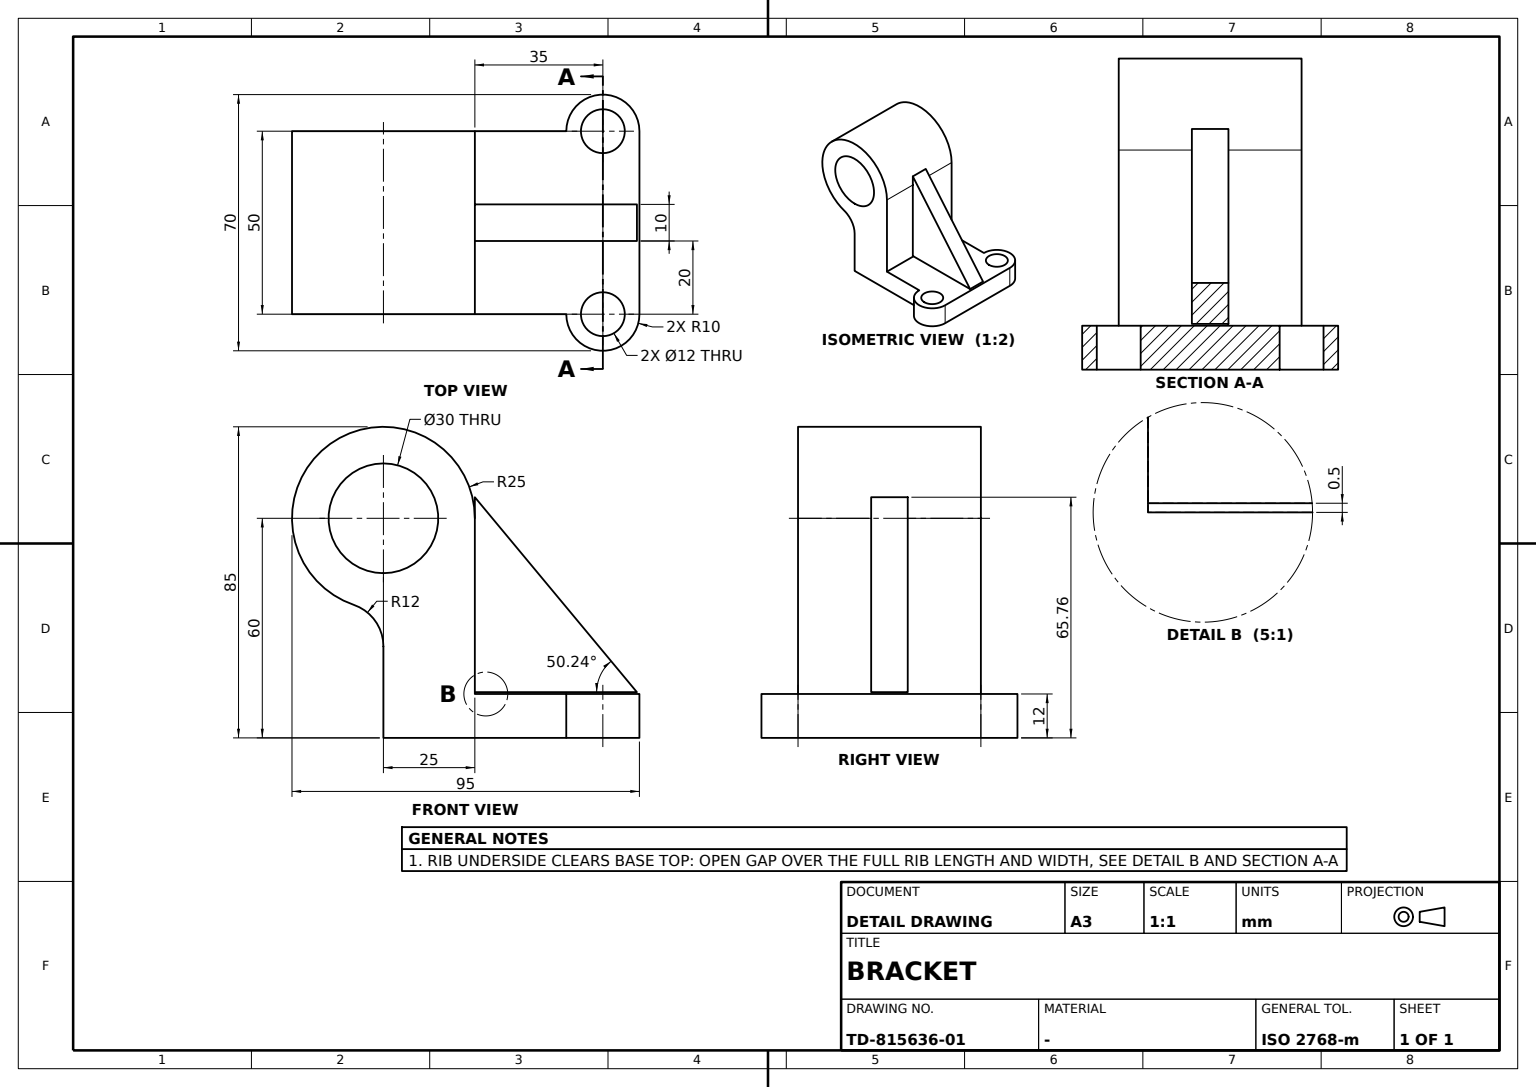
CATIA V5 part; units mm, degrees
sketch "Sketch1" plane through (0, 0, 0) normal (1, 0, 0) x (0, 1, 0)
  point P0 (0, 54)
  line L0 (0, 54) -> (0, 6)
  line L1 (0, 6) -> (45, 6)
  point P1 (45, 6)
  line L2 (45, 6) -> (45, -6)
  point P2 (45, -6)
  line L3 (45, -6) -> (-25, -6)
  line L4 (-25, -6) -> (-25, 19)
  point P3 (-25, 54)
  circle A0 centre (-25, 54) radius 15
  arc A1 (0, 54) -> (-33.1081, 30.3514) centre (-25, 54) ccw
  point P4 (0, 54)
  arc A2 (-33.1081, 30.3514) -> (-25, 19) centre (-37, 19) cw
  point P5 (0, 54)
  dimension "length L2" = 12
  dimension "distance L4 L0" = 25
  dimension "length L3" = 70
  dimension "radius A1" = 25
  dimension "radius A0" = 15
  dimension "radius A2" = 12
  dimension "distance P3 L3" = 60
  constraint vertical L0 y-axis
  constraint vertical L2 y-axis
  constraint vertical L4 y-axis
  constraint horizontal L1 x-axis
  constraint horizontal L3 x-axis
  constraint coincidence A1 P4
  constraint coincidence P4 y-axis
  constraint coincidence L4 P3
  constraint coincidence P4 P0
  constraint coincidence P0 P5
  constraint symmetry P1 P2 x-axis
  constraint tangency A2 A1
  constraint tangency A2 L4
extrude "Pad1" add sketch "Sketch1" along normal blind 50
sketch "Sketch2" plane through (0, 0, 6) normal (0, 0, 1) x (1, 0, 0)
  circle A0 centre (50, 35) radius 10
  point P0 (50, 35)
  circle A1 centre (0, 35) radius 10
  point P1 (0, 35)
  line L0 (50, 45) -> (50, 0) construction
  line L1 (0, 45) -> (50, 45) construction
  line L2 (0, 45) -> (50, 45) construction
  dimension "radius A0" = 10
  dimension "radius A1" = 10
  dimension "distance L1 P0" = 10
  dimension "distance L2 P1" = 10
  constraint coincidence P1 y-axis
  constraint coincidence P0 L0
extrude "Pad2" add sketch "Sketch2" against normal blind 12
sketch "Sketch3" plane through (0, 0, 6) normal (0, 0, 1) x (1, 0, 0)
  circle A0 centre (0, 35) radius 6
  point P0 (0, 35)
  circle A1 centre (50, 35) radius 6
  point P1 (50, 35)
  circle A2 centre (0, 35) radius 10 construction
  circle A3 centre (50, 35) radius 10 construction
  dimension "radius A1" = 6
  dimension "radius A0" = 6
  dimension "distance P0 P1" = 50
  dimension "distance P0 A2" = 10
  dimension "distance P1 A3 x axis" = 10
  constraint coincidence P0 y-axis
extrude "Pocket1" cut sketch "Sketch3" against normal blind 12
ref_plane "Plane1" through (25, 0, 0) normal (1, 0, 0) x (0, 1, 0)
sketch "Sketch4" plane through (25, 0, 0) normal (1, 0, 0) x (0, 1, 0)
  point P0 (0, 59.7595)
  line L0 (0, 59.7595) -> (0, 6.5)
  line L1 (0, 6.5) -> (44.315, 6.5)
  line L2 (44.315, 6.5) -> (0, 59.7595)
  line L3 (25, 6) -> (45, 6) construction
  dimension "distance L1 L3" = 0.5
  constraint coincidence P0 y-axis
  constraint vertical L0 y-axis
  constraint horizontal L1 x-axis
extrude "Pad3" add sketch "Sketch4" along normal mid plane 10
